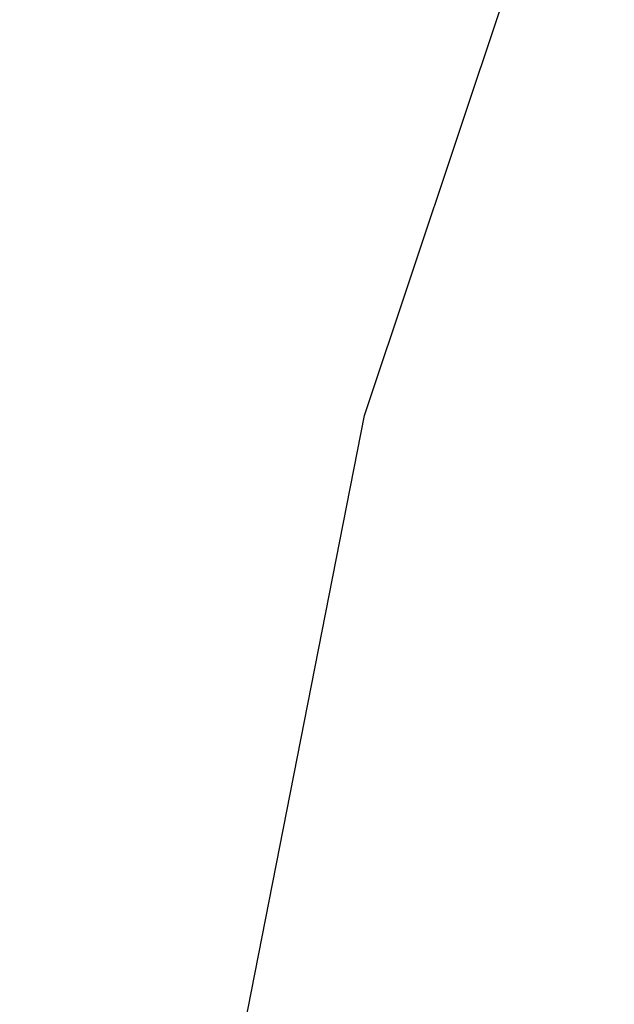
# Model space of a CAD drawing. Units: inches. Extents: x 3590 to 5167, y 65 to 1917.
# Tile 81 of 100: x 5050.9101 to 5051.162, y 1788.6144 to 1789.0318. Entities that reach past the tile are written whole.
import ezdxf

# ---------------------------------------------------------------- set-up
doc = ezdxf.new("R2010")
doc.units = ezdxf.units.IN
for name, color, linetype, lineweight in [('A-ANNO-DIMS', 2, 'Continuous', 18), ('A-FLOR-PATT', 8, 'Continuous', 13), ('L-PLNT', 94, 'Continuous', 18)]:
    doc.layers.add(name, color=color, linetype=linetype, lineweight=lineweight)
doc.layers.add('DIENHOA', color=3, linetype='Continuous')
doc.styles.get("Standard").update_dxf_attribs({"font": 'arial.ttf'})
doc.dimstyles.new('ISO-25', dxfattribs={"dimtxt": 9, "dimasz": 2.5, "dimexe": 1.25, "dimexo": 0.625, "dimtad": 1, "dimdec": 1, "dimlunit": 3, "dimtxsty": 'Standard', "dimcen": 2.5, "dimadec": 0, "dimazin": 0, "dimtfac": 1, "dimtdec": 1, "dimtmove": 0, "dimatfit": 3, "dimfxl": 1, "dimarcsym": 0})

# ---------------------------------------------------------------- blocks, each defined once
blk = doc.blocks.new('Cay03_mb')
at = {"layer": 'DIENHOA'}
for p, q in [((25.486, 374.333), (48.564, 443.581)), ((9.944, 295.252), (25.486, 374.333))]:
    blk.add_line(p, q, dxfattribs=at)
blk = doc.blocks.new('*D323')
at = {"layer": 'A-ANNO-DIMS', "color": 0, "lineweight": -2, "transparency": 16777216}
for p, q in [((5069.17227, 1795.21603), (5069.17227, 1874.95034)), ((5065.43703, 1795.21603), (5070.42227, 1795.21603)), ((5069.17227, 1769.30924), (5069.17227, 1792.71603)), ((5065.43703, 1766.80924), (5070.42227, 1766.80924))]:
    blk.add_line(p, q, dxfattribs=at)
at = {"layer": 'A-ANNO-DIMS', "color": 0, "transparency": 16777216}
for points in [[(5068.75561, 1792.71603), (5069.58894, 1792.71603), (5069.17227, 1795.21603)], [(5068.75561, 1769.30924), (5069.58894, 1769.30924), (5069.17227, 1766.80924)]]:
    blk.add_solid(points, dxfattribs=at)
at = {"layer": 'Defpoints', "color": 0, "transparency": 16777216}
for p in [(5064.81203, 1795.21603), (5069.17227, 1795.21603), (5064.81203, 1766.80924)]:
    blk.add_point(p, dxfattribs=at)
at = {"layer": 'A-ANNO-DIMS', "color": 0, "transparency": 16777216, "insert": (5063.89379, 1836.33318), "char_height": 9, "attachment_point": 5, "rotation": 90}
blk.add_mtext('2\'-4 1/2" TYP.', dxfattribs=at)

msp = doc.modelspace()

# ---------------------------------------------------------------- hatches: boundary and pattern name
at = {"layer": 'A-FLOR-PATT', "transparency": 33554687}
h = msp.add_hatch(dxfattribs=at)
h.set_pattern_fill('AR-HBONE', color=256, scale=0.2)
h.set_pattern_definition([(45, (-588.972, 0), (0, 28.73682), [60.96, -20.32]), (135, (-574.604, 14.368), (3e-15, 28.73682), [60.96, -20.32])])
h.paths.add_polyline_path([(5071.27403, 1796.99898), (4933.27403, 1796.99898), (4933.27403, 1753.99898), (4962.77403, 1753.99898, -0.414214), (4928.77403, 1719.99898), (4933.27403, 1718.99898), (4933.27403, 1334.99898), (5071.27403, 1334.99898)])
h.paths.add_polyline_path([(4951.78002, 1521.0767), (4951.7151, 1521.0404), (4951.56345, 1520.89532)], flags=16)
h.paths.add_polyline_path([(4952.267, 1521.37645), (4952.1977, 1521.37111), (4952.19823, 1521.35558)], flags=0)
h.paths.add_polyline_path([(4967.05076, 1529.72832), (4965.23122, 1528.69444), (4963.41109, 1527.71401), (4961.75649, 1526.85081), (4963.58887, 1527.44938), (4964.03555, 1527.47802), (4962.9755, 1527.24902), (4961.76022, 1526.85203), (4959.79219, 1525.83406), (4958.00498, 1524.89483), (4956.24031, 1523.92961), (4954.50395, 1522.91854), (4954.1294, 1522.68163), (4953.36051, 1521.99688), (4953.36558, 1521.99754), (4953.605, 1522.06367), (4955.10605, 1522.76083), (4956.92108, 1523.43405), (4958.67784, 1523.91513), (4960.35834, 1524.20036), (4961.94456, 1524.28606), (4964.17144, 1524.10849), (4965.95752, 1523.30903), (4963.86273, 1522.97565), (4965.18742, 1522.49898), (4963.36614, 1522.49715), (4961.54526, 1522.48682), (4959.76359, 1522.46077), (4958.30414, 1522.4188), (4957.97356, 1522.38829), (4956.30692, 1522.2324), (4954.71821, 1522.07143), (4953.25077, 1521.89915), (4953.52509, 1521.62277), (4954.33087, 1521.37883), (4956.24263, 1521.22987), (4958.03913, 1520.92952), (4959.68424, 1520.48339), (4961.16007, 1519.89569), (4963.10699, 1518.80022), (4964.39286, 1517.32518), (4962.97306, 1517.72596), (4964.55841, 1516.66059), (4965.40664, 1515.70779), (4963.50733, 1516.32179), (4961.67995, 1517.0051), (4959.93478, 1517.74489), (4958.2821, 1518.52833), (4956.73216, 1519.34257), (4955.29527, 1520.17478), (4954.67155, 1520.57237), (4954.51279, 1520.6271), (4955.65848, 1519.31837), (4956.70263, 1517.98232), (4957.64403, 1516.64663), (4958.48545, 1515.33439), (4959.54998, 1513.52398), (4960.43768, 1511.76936), (4958.84107, 1513.6196), (4957.45175, 1515.3249), (4955.8186, 1517.45855), (4956.66537, 1515.44764), (4957.11109, 1513.92292), (4957.44681, 1511.71434), (4957.07641, 1509.79288), (4956.53757, 1511.1103), (4955.99231, 1512.56892), (4955.44448, 1514.12509), (4954.89794, 1515.73518), (4954.35653, 1517.35553), (4953.82412, 1518.94251), (4953.30455, 1520.45247), (4953.06452, 1521.11563), (4952.97143, 1521.14607), (4952.94932, 1521.08646), (4952.72981, 1520.19905), (4953.3698, 1518.02364), (4953.75708, 1516.37279), (4954.05124, 1514.76538), (4954.26449, 1513.22121), (4954.47124, 1511.13121), (4954.4971, 1510.40174), (4954.40903, 1511.76006), (4954.26449, 1513.22121), (4954.05124, 1514.76538), (4953.75708, 1516.37279), (4953.3698, 1518.02364), (4952.87718, 1519.69813), (4952.7161, 1520.1412), (4952.53301, 1519.05871), (4952.37428, 1517.78881), (4952.21925, 1516.31167), (4952.04598, 1514.59986), (4951.83253, 1512.62598), (4951.55697, 1510.36259), (4951.20331, 1512.16818), (4950.85168, 1514.33931), (4950.98529, 1516.37594), (4951.6596, 1518.28625), (4952.59261, 1520.48085), (4952.35664, 1521.1299), (4951.85502, 1520.32753), (4950.83901, 1518.90828), (4949.77675, 1517.58658), (4948.91554, 1516.61731), (4948.11099, 1515.2561), (4947.0891, 1513.55389), (4945.88937, 1511.61495), (4946.32587, 1513.40232), (4946.5624, 1514.24913), (4945.52771, 1513.32668), (4944.58105, 1512.53126), (4946.01774, 1514.50825), (4947.2044, 1516.04763), (4947.89331, 1517.31331), (4949.30686, 1518.76446), (4950.41417, 1519.76716), (4950.45131, 1519.80628), (4952.267, 1521.37645), (4951.64457, 1521.49317), (4950.40371, 1521.17954), (4948.04447, 1520.35868), (4946.11863, 1519.45198), (4944.57182, 1518.47484), (4943.34962, 1517.44265), (4941.99695, 1515.91971), (4941.66146, 1515.27475), (4942.81332, 1516.98973), (4944.57182, 1518.47484), (4946.11863, 1519.45198), (4948.04447, 1520.35868), (4950.40371, 1521.17954), (4951.64457, 1521.49317), (4949.64678, 1521.86781), (4948.59979, 1521.75633), (4947.12629, 1521.5699), (4945.42015, 1521.34763), (4943.44969, 1521.10462), (4941.18319, 1520.85596), (4942.86028, 1521.61265), (4943.87308, 1522.03014), (4942.95216, 1521.9093), (4941.40968, 1521.48512), (4939.54287, 1520.67019), (4938.96775, 1520.2255), (4940.73284, 1521.29899), (4942.95216, 1521.9093), (4943.70184, 1522.00767), (4945.89419, 1522.69998), (4947.56488, 1522.71399), (4948.92086, 1522.56573), (4951.13144, 1522.18271), (4950.97062, 1522.2969), (4948.12924, 1523.00563), (4946.03496, 1523.70671), (4944.23235, 1524.52143), (4942.70692, 1525.46111), (4941.44419, 1526.53707), (4940.42968, 1527.76062), (4939.6489, 1529.14306), (4941.42091, 1528.12232), (4943.14742, 1527.13248), (4944.84093, 1526.17457), (4946.51394, 1525.24959), (4948.17893, 1524.35855), (4948.36457, 1524.26336), (4946.47531, 1526.04459), (4945.18083, 1527.54042), (4944.19039, 1529.03339), (4943.49559, 1530.53985), (4943.27808, 1531.3597), (4942.49849, 1531.91903), (4943.11353, 1531.76249), (4942.95927, 1533.6586), (4944.13953, 1531.9886), (4944.61171, 1531.32339), (4946.20163, 1530.46341), (4947.48567, 1529.50925), (4948.79027, 1528.22649), (4950.36754, 1526.23746), (4949.48547, 1528.15549), (4948.85128, 1530.12254), (4948.49054, 1532.04127), (4948.38105, 1533.91822), (4948.50062, 1535.7599), (4948.82704, 1537.57284), (4949.41803, 1535.56526), (4949.95684, 1533.56932), (4950.46414, 1531.5861), (4950.96058, 1529.6167), (4951.3911, 1527.95448), (4951.72352, 1530.68689), (4952.20106, 1532.57994), (4952.88914, 1534.32964), (4953.77035, 1535.95123), (4954.82726, 1537.45995), (4954.52145, 1535.38966), (4954.27314, 1533.93684), (4955.57999, 1535.6627), (4956.74758, 1536.73859), (4956.15852, 1534.78029), (4955.58917, 1532.87334), (4955.04336, 1531.00581), (4954.52493, 1529.16576), (4954.03771, 1527.34127), (4953.63833, 1525.73298), (4953.61143, 1525.58564), (4953.39805, 1524.16565), (4953.38219, 1524.00887), (4954.06955, 1525.47563), (4954.91212, 1527.02173), (4956.13627, 1528.89351), (4957.84668, 1530.57701), (4959.37601, 1531.54014), (4958.25596, 1530.10398), (4957.14284, 1528.66291), (4956.06626, 1527.24305), (4955.05579, 1525.87054), (4954.14104, 1524.57149), (4953.35159, 1523.37204), (4953.31079, 1523.30299), (4953.27253, 1522.92478), (4953.26102, 1522.38213), (4954.1031, 1523.37273), (4954.63005, 1524.28376), (4955.96149, 1526.35767), (4957.23002, 1528.12969), (4958.42057, 1529.60864), (4960.03671, 1531.36792), (4961.3736, 1532.3752), (4962.1015, 1532.77), (4961.06994, 1531.06113), (4959.98733, 1529.43811), (4958.86851, 1527.90803), (4958.15046, 1527.00742), (4959.80291, 1528.00314), (4961.58854, 1528.79257), (4963.39087, 1529.32783), (4965.21118, 1529.63205)], flags=16)
h.paths.add_polyline_path([(4962.94387, 1523.18187), (4961.10714, 1523.42192), (4960.39205, 1523.36158), (4962.34964, 1523.33061)], flags=0)
h.paths.add_polyline_path([(5049.54129, 1584.55089), (5049.47636, 1584.51458), (5049.32471, 1584.3695)], flags=16)
h.paths.add_polyline_path([(5050.02827, 1584.85063), (5049.95897, 1584.84529), (5049.95949, 1584.82976)], flags=0)
h.paths.add_polyline_path([(5042.33308, 1581.94902), (5043.8799, 1582.92616), (5045.80573, 1583.83286), (5048.16498, 1584.65372), (5049.40583, 1584.96736), (5047.40804, 1585.34199), (5046.36106, 1585.23052), (5044.88755, 1585.04408), (5043.18142, 1584.82181), (5041.21095, 1584.5788), (5038.94446, 1584.33014), (5040.62155, 1585.08683), (5041.63434, 1585.50432), (5040.71343, 1585.38348), (5039.17095, 1584.9593), (5037.30414, 1584.14438), (5036.72901, 1583.69969), (5038.4941, 1584.77317), (5040.71343, 1585.38348), (5041.4631, 1585.48185), (5043.65545, 1586.17416), (5045.32615, 1586.18818), (5046.68212, 1586.03992), (5048.8927, 1585.6569), (5048.73188, 1585.77108), (5045.89051, 1586.47981), (5043.79622, 1587.18089), (5041.99361, 1587.99561), (5040.46818, 1588.9353), (5039.20546, 1590.01125), (5038.19095, 1591.2348), (5037.41016, 1592.61725), (5039.18217, 1591.5965), (5040.90868, 1590.60667), (5042.6022, 1589.64876), (5044.2752, 1588.72378), (5045.94019, 1587.83274), (5046.12584, 1587.73754), (5044.23658, 1589.51878), (5042.9421, 1591.01461), (5041.95166, 1592.50757), (5041.25685, 1594.01403), (5041.03935, 1594.83388), (5040.25976, 1595.39321), (5040.8748, 1595.23667), (5040.72054, 1597.13279), (5041.9008, 1595.46278), (5042.37297, 1594.79758), (5043.96289, 1593.93759), (5045.24694, 1592.98344), (5046.55153, 1591.70068), (5048.12881, 1589.71164), (5047.24673, 1591.62967), (5046.61254, 1593.59672), (5046.2518, 1595.51546), (5046.14232, 1597.3924), (5046.26189, 1599.23408), (5046.5883, 1601.04703), (5047.17929, 1599.03944), (5047.71811, 1597.0435), (5048.22541, 1595.06028), (5048.72184, 1593.09089), (5049.15237, 1591.42866), (5049.48478, 1594.16107), (5049.96233, 1596.05412), (5050.65041, 1597.80382), (5051.53161, 1599.42541), (5052.58852, 1600.93414), (5052.28271, 1598.86384), (5052.03441, 1597.41102), (5053.34126, 1599.13689), (5054.50884, 1600.21277), (5053.91979, 1598.25447), (5053.35044, 1596.34752), (5052.80463, 1594.47999), (5052.2862, 1592.63995), (5051.79898, 1590.81546), (5051.39959, 1589.20716), (5051.3727, 1589.05983), (5051.15931, 1587.63984), (5051.14346, 1587.48305), (5051.83082, 1588.94982), (5052.67339, 1590.49592), (5053.89754, 1592.3677), (5055.60794, 1594.05119), (5057.13728, 1595.01432), (5056.01722, 1593.57817), (5054.90411, 1592.1371), (5053.82752, 1590.71724), (5052.81705, 1589.34472), (5051.9023, 1588.04567), (5051.11286, 1586.84622), (5051.07205, 1586.77718), (5051.03379, 1586.39896), (5051.02228, 1585.85631), (5051.86437, 1586.84692), (5052.39131, 1587.75794), (5053.72275, 1589.83185), (5054.99128, 1591.60387), (5056.18183, 1593.08282), (5057.79798, 1594.84211), (5059.13486, 1595.84938), (5059.86276, 1596.24419), (5058.83121, 1594.53531), (5057.7486, 1592.9123), (5056.62978, 1591.38221), (5055.91173, 1590.4816), (5057.56418, 1591.47732), (5059.34981, 1592.26675), (5061.15214, 1592.80202), (5062.97245, 1593.10624), (5064.81203, 1593.20251), (5062.99248, 1592.16863), (5061.17235, 1591.18819), (5059.51775, 1590.325), (5061.35014, 1590.92356), (5061.79682, 1590.95221), (5060.73676, 1590.7232), (5059.52148, 1590.32622), (5057.55345, 1589.30825), (5055.76625, 1588.36901), (5054.00157, 1587.40379), (5052.26521, 1586.39273), (5051.89067, 1586.15581), (5051.12177, 1585.47106), (5051.12684, 1585.47172), (5051.36627, 1585.53786), (5052.86732, 1586.23502), (5054.68234, 1586.90824), (5056.4391, 1587.38931), (5058.1196, 1587.67454), (5059.70582, 1587.76024), (5061.93271, 1587.58268), (5063.71878, 1586.78321), (5061.62399, 1586.44983), (5062.94869, 1585.97317), (5061.12741, 1585.97133), (5059.30653, 1585.961), (5057.52486, 1585.93496), (5056.06541, 1585.89299), (5055.73482, 1585.86247), (5054.06819, 1585.70658), (5052.47947, 1585.54561), (5051.01204, 1585.37333), (5051.28635, 1585.09695), (5052.09214, 1584.85301), (5054.00389, 1584.70406), (5055.8004, 1584.4037), (5057.44551, 1583.95757), (5058.92133, 1583.36987), (5060.86825, 1582.27441), (5062.15413, 1580.79937), (5060.73433, 1581.20015), (5062.31967, 1580.13477), (5063.1679, 1579.18198), (5061.2686, 1579.79597), (5059.44122, 1580.47928), (5057.69605, 1581.21908), (5056.04336, 1582.00251), (5054.49343, 1582.81675), (5053.05653, 1583.64897), (5052.43281, 1584.04656), (5052.27405, 1584.10128), (5053.41974, 1582.79255), (5054.4639, 1581.4565), (5055.40529, 1580.12081), (5056.24672, 1578.80858), (5057.31125, 1576.99816), (5058.19895, 1575.24354), (5056.60234, 1577.09378), (5055.21301, 1578.79908), (5053.57987, 1580.93274), (5054.42664, 1578.92183), (5054.87235, 1577.3971), (5055.20808, 1575.18852), (5054.83767, 1573.26706), (5054.29883, 1574.58448), (5053.75357, 1576.0431), (5053.20575, 1577.59927), (5052.6592, 1579.20936), (5052.1178, 1580.82971), (5051.58538, 1582.41669), (5051.06582, 1583.92666), (5050.82578, 1584.58981), (5050.7327, 1584.62025), (5050.71058, 1584.56064), (5050.49108, 1583.67323), (5051.13107, 1581.49782), (5051.51835, 1579.84698), (5051.8125, 1578.23957), (5052.02575, 1576.69539), (5052.23251, 1574.6054), (5052.25836, 1573.87593), (5052.1703, 1575.23424), (5052.02575, 1576.69539), (5051.8125, 1578.23957), (5051.51835, 1579.84698), (5051.13107, 1581.49782), (5050.63844, 1583.17231), (5050.47736, 1583.61538), (5050.29428, 1582.53289), (5050.13554, 1581.26299), (5049.98051, 1579.78585), (5049.80724, 1578.07405), (5049.59379, 1576.10016), (5049.31823, 1573.83678), (5048.96458, 1575.64237), (5048.61294, 1577.8135), (5048.74656, 1579.85012), (5049.42086, 1581.76043), (5050.35388, 1583.95503), (5050.1179, 1584.60408), (5049.61629, 1583.80172), (5048.60027, 1582.38246), (5047.53801, 1581.06076), (5046.67681, 1580.09149), (5045.87225, 1578.73029), (5044.85036, 1577.02808), (5043.65063, 1575.08913), (5044.08713, 1576.8765), (5044.32366, 1577.72331), (5043.28898, 1576.80086), (5042.34232, 1576.00545), (5043.779, 1577.98243), (5044.96566, 1579.52182), (5045.65457, 1580.78749), (5047.06813, 1582.23865), (5048.17543, 1583.24134), (5048.21258, 1583.28047), (5050.02827, 1584.85063), (5049.40583, 1584.96736), (5048.16498, 1584.65372), (5045.80573, 1583.83286), (5043.8799, 1582.92616), (5042.33308, 1581.94902), (5041.11088, 1580.91684), (5039.75821, 1579.39389), (5039.42272, 1578.74894), (5040.57458, 1580.46391)], flags=16)
h.paths.add_polyline_path([(4954.79872, 1533.12029), (4954.26249, 1532.07935), (4953.83112, 1530.93464), (4953.50472, 1529.63602), (4953.28338, 1528.13331), (4953.16721, 1526.37637), (4953.15631, 1524.31504), (4953.27669, 1521.23629), (4952.80168, 1521.84177), (4951.55695, 1521.99789), (4950.97575, 1521.9613), (4952.66059, 1521.94097), (4952.80168, 1521.84177), (4953.15249, 1523.59258), (4953.16721, 1526.37637), (4953.28338, 1528.13331), (4953.60929, 1530.34598), (4954.45558, 1532.59174)], flags=0)
h.paths.add_polyline_path([(5050.56294, 1585.31596), (5049.31822, 1585.47208), (5048.73702, 1585.43548), (5050.42186, 1585.41516), (5050.56294, 1585.31596), (5050.91375, 1587.06676), (5050.92848, 1589.85056), (5051.04465, 1591.6075), (5051.37055, 1593.82017), (5052.21684, 1596.06593), (5052.55999, 1596.59447), (5052.02375, 1595.55353), (5051.59238, 1594.40883), (5051.26598, 1593.1102), (5051.04465, 1591.6075), (5050.92848, 1589.85056), (5050.91757, 1587.78922), (5051.03795, 1584.71048)], flags=0)
h.paths.add_polyline_path([(5058.15332, 1586.83576), (5060.11091, 1586.80479), (5060.70514, 1586.65605), (5058.8684, 1586.8961)], flags=0)
h.paths.add_polyline_path([(5049.54129, 1430.93611), (5049.47636, 1430.8998), (5049.32471, 1430.75472)], flags=16)
h.paths.add_polyline_path([(5050.02827, 1431.23585), (5049.95897, 1431.23051), (5049.95949, 1431.21498)], flags=0)
h.paths.add_polyline_path([(5046.5883, 1447.43225), (5047.17929, 1445.42467), (5047.71811, 1443.42872), (5048.22541, 1441.4455), (5048.72184, 1439.47611), (5049.15237, 1437.81388), (5049.48478, 1440.5463), (5049.96233, 1442.43934), (5050.65041, 1444.18904), (5051.53161, 1445.81063), (5052.58852, 1447.31936), (5052.28271, 1445.24906), (5052.03441, 1443.79624), (5053.34126, 1445.52211), (5054.50884, 1446.59799), (5053.91979, 1444.63969), (5053.35044, 1442.73274), (5052.80463, 1440.86521), (5052.2862, 1439.02517), (5051.79898, 1437.20068), (5051.39959, 1435.59238), (5051.3727, 1435.44505), (5051.15931, 1434.02506), (5051.14346, 1433.86828), (5051.83082, 1435.33504), (5052.67339, 1436.88114), (5053.89754, 1438.75292), (5055.60794, 1440.43641), (5057.13728, 1441.39954), (5056.01722, 1439.96339), (5054.90411, 1438.52232), (5053.82752, 1437.10246), (5052.81705, 1435.72994), (5051.9023, 1434.4309), (5051.11286, 1433.23145), (5051.07205, 1433.1624), (5051.03379, 1432.78418), (5051.02228, 1432.24153), (5051.86437, 1433.23214), (5052.39131, 1434.14316), (5053.72275, 1436.21707), (5054.99128, 1437.98909), (5056.18183, 1439.46805), (5057.79798, 1441.22733), (5059.13486, 1442.23461), (5059.86276, 1442.62941), (5058.83121, 1440.92053), (5057.7486, 1439.29752), (5056.62978, 1437.76743), (5055.91173, 1436.86682), (5057.56418, 1437.86255), (5059.34981, 1438.65197), (5061.15214, 1439.18724), (5062.97245, 1439.49146), (5064.81203, 1439.58773), (5062.99248, 1438.55385), (5061.17235, 1437.57342), (5059.51775, 1436.71022), (5061.35014, 1437.30879), (5061.79682, 1437.33743), (5060.73676, 1437.10842), (5059.52148, 1436.71144), (5057.55345, 1435.69347), (5055.76625, 1434.75423), (5054.00157, 1433.78901), (5052.26521, 1432.77795), (5051.89067, 1432.54103), (5051.12177, 1431.85628), (5051.12684, 1431.85694), (5051.36627, 1431.92308), (5052.86732, 1432.62024), (5054.68234, 1433.29346), (5056.4391, 1433.77453), (5058.1196, 1434.05976), (5059.70582, 1434.14546), (5061.93271, 1433.9679), (5063.71878, 1433.16843), (5061.62399, 1432.83505), (5062.94869, 1432.35839), (5061.12741, 1432.35655), (5059.30653, 1432.34623), (5057.52486, 1432.32018), (5056.06541, 1432.27821), (5055.73482, 1432.24769), (5054.06819, 1432.09181), (5052.47947, 1431.93083), (5051.01204, 1431.75856), (5051.28635, 1431.48218), (5052.09214, 1431.23823), (5054.00389, 1431.08928), (5055.8004, 1430.78892), (5057.44551, 1430.34279), (5058.92133, 1429.75509), (5060.86825, 1428.65963), (5062.15413, 1427.18459), (5060.73433, 1427.58537), (5062.31967, 1426.52), (5063.1679, 1425.5672), (5061.2686, 1426.18119), (5059.44122, 1426.86451), (5057.69605, 1427.6043), (5056.04336, 1428.38773), (5054.49343, 1429.20197), (5053.05653, 1430.03419), (5052.43281, 1430.43178), (5052.27405, 1430.48651), (5053.41974, 1429.17777), (5054.4639, 1427.84172), (5055.40529, 1426.50603), (5056.24672, 1425.1938), (5057.31125, 1423.38338), (5058.19895, 1421.62877), (5056.60234, 1423.479), (5055.21301, 1425.1843), (5053.57987, 1427.31796), (5054.42664, 1425.30705), (5054.87235, 1423.78233), (5055.20808, 1421.57374), (5054.83767, 1419.65228), (5054.29883, 1420.9697), (5053.75357, 1422.42832), (5053.20575, 1423.9845), (5052.6592, 1425.59458), (5052.1178, 1427.21493), (5051.58538, 1428.80191), (5051.06582, 1430.31188), (5050.82578, 1430.97503), (5050.7327, 1431.00547), (5050.71058, 1430.94586), (5050.49108, 1430.05845), (5051.13107, 1427.88305), (5051.51835, 1426.2322), (5051.8125, 1424.62479), (5052.02575, 1423.08061), (5052.23251, 1420.99062), (5052.25836, 1420.26115), (5052.1703, 1421.61947), (5052.02575, 1423.08061), (5051.8125, 1424.62479), (5051.51835, 1426.2322), (5051.13107, 1427.88305), (5050.63844, 1429.55753), (5050.47736, 1430.0006), (5050.29428, 1428.91811), (5050.13554, 1427.64821), (5049.98051, 1426.17107), (5049.80724, 1424.45927), (5049.59379, 1422.48539), (5049.31823, 1420.222), (5048.96458, 1422.02759), (5048.61294, 1424.19872), (5048.74656, 1426.23534), (5049.42086, 1428.14565), (5050.35388, 1430.34025), (5050.1179, 1430.98931), (5049.61629, 1430.18694), (5048.60027, 1428.76768), (5047.53801, 1427.44598), (5046.67681, 1426.47671), (5045.87225, 1425.11551), (5044.85036, 1423.4133), (5043.65063, 1421.47435), (5044.08713, 1423.26172), (5044.32366, 1424.10854), (5043.28898, 1423.18608), (5042.34232, 1422.39067), (5043.779, 1424.36765), (5044.96566, 1425.90704), (5045.65457, 1427.17272), (5047.06813, 1428.62387), (5048.17543, 1429.62657), (5048.21258, 1429.66569), (5050.02827, 1431.23585), (5049.40583, 1431.35258), (5048.16498, 1431.03894), (5045.80573, 1430.21809), (5043.8799, 1429.31139), (5042.33308, 1428.33424), (5041.11088, 1427.30206), (5039.75821, 1425.77911), (5039.42272, 1425.13416), (5040.57458, 1426.84914), (5042.33308, 1428.33424), (5043.8799, 1429.31139), (5045.80573, 1430.21809), (5048.16498, 1431.03894), (5049.40583, 1431.35258), (5047.40804, 1431.72722), (5046.36106, 1431.61574), (5044.88755, 1431.42931), (5043.18142, 1431.20704), (5041.21095, 1430.96402), (5038.94446, 1430.71536), (5040.62155, 1431.47205), (5041.63434, 1431.88954), (5040.71343, 1431.76871), (5039.17095, 1431.34453), (5037.30414, 1430.5296), (5036.72901, 1430.08491), (5038.4941, 1431.1584), (5040.71343, 1431.76871), (5041.4631, 1431.86707), (5043.65545, 1432.55939), (5045.32615, 1432.5734), (5046.68212, 1432.42514), (5048.8927, 1432.04212), (5048.73188, 1432.1563), (5045.89051, 1432.86503), (5043.79622, 1433.56611), (5041.99361, 1434.38083), (5040.46818, 1435.32052), (5039.20546, 1436.39648), (5038.19095, 1437.62002), (5037.41016, 1439.00247), (5039.18217, 1437.98172), (5040.90868, 1436.99189), (5042.6022, 1436.03398), (5044.2752, 1435.109), (5045.94019, 1434.21796), (5046.12584, 1434.12276), (5044.23658, 1435.904), (5042.9421, 1437.39983), (5041.95166, 1438.8928), (5041.25685, 1440.39925), (5041.03935, 1441.2191), (5040.25976, 1441.77844), (5040.8748, 1441.62189), (5040.72054, 1443.51801), (5041.9008, 1441.848), (5042.37297, 1441.1828), (5043.96289, 1440.32282), (5045.24694, 1439.36866), (5046.55153, 1438.0859), (5048.12881, 1436.09686), (5047.24673, 1438.01489), (5046.61254, 1439.98195), (5046.2518, 1441.90068), (5046.14232, 1443.77762), (5046.26189, 1445.6193)], flags=16)
h.paths.add_polyline_path([(5052.38176, 1444.25496), (5051.62263, 1442.77987), (5052.02375, 1441.93875), (5052.55999, 1442.9797)], flags=0)
h.paths.add_polyline_path([(5050.56294, 1431.70118), (5049.31822, 1431.8573), (5048.73702, 1431.82071), (5050.42186, 1431.80038)], flags=0)
h.paths.add_polyline_path([(5058.15332, 1433.22098), (5060.11091, 1433.19001), (5060.70514, 1433.04127), (5058.8684, 1433.28132)], flags=0)
h.paths.add_polyline_path([(5049.54129, 1352.28535), (5049.47636, 1352.24904), (5049.32471, 1352.10396)], flags=16)
h.paths.add_polyline_path([(5050.02827, 1352.58509), (5049.95897, 1352.57975), (5049.95949, 1352.56422)], flags=0)
h.paths.add_polyline_path([(5046.5883, 1368.78149), (5047.17929, 1366.7739), (5047.71811, 1364.77796), (5048.22541, 1362.79474), (5048.72184, 1360.82534), (5049.15237, 1359.16312), (5049.48478, 1361.89553), (5049.96233, 1363.78858), (5050.65041, 1365.53828), (5051.53161, 1367.15987), (5052.58852, 1368.6686), (5052.28271, 1366.5983), (5052.03441, 1365.14548), (5053.34126, 1366.87135), (5054.50884, 1367.94723), (5053.91979, 1365.98893), (5053.35044, 1364.08198), (5052.80463, 1362.21445), (5052.2862, 1360.37441), (5051.79898, 1358.54992), (5051.39959, 1356.94162), (5051.3727, 1356.79428), (5051.15931, 1355.37429), (5051.14346, 1355.21751), (5051.83082, 1356.68428), (5052.67339, 1358.23037), (5053.89754, 1360.10216), (5055.60794, 1361.78565), (5057.13728, 1362.74878), (5056.01722, 1361.31262), (5054.90411, 1359.87155), (5053.82752, 1358.4517), (5052.81705, 1357.07918), (5051.9023, 1355.78013), (5051.11286, 1354.58068), (5051.07205, 1354.51164), (5051.03379, 1354.13342), (5051.02228, 1353.59077), (5051.86437, 1354.58137), (5052.39131, 1355.4924), (5053.72275, 1357.56631), (5054.99128, 1359.33833), (5056.18183, 1360.81728), (5057.79798, 1362.57656), (5059.13486, 1363.58384), (5059.86276, 1363.97864), (5058.83121, 1362.26977), (5057.7486, 1360.64675), (5056.62978, 1359.11667), (5055.91173, 1358.21606), (5057.56418, 1359.21178), (5059.34981, 1360.00121), (5061.15214, 1360.53648), (5062.97245, 1360.84069), (5064.81203, 1360.93697), (5062.99248, 1359.90308), (5061.17235, 1358.92265), (5059.51775, 1358.05946), (5061.35014, 1358.65802), (5061.79682, 1358.68666), (5060.73676, 1358.45766), (5059.52148, 1358.06068), (5057.55345, 1357.0427), (5055.76625, 1356.10347), (5054.00157, 1355.13825), (5052.26521, 1354.12718), (5051.89067, 1353.89027), (5051.12177, 1353.20552), (5051.12684, 1353.20618), (5051.36627, 1353.27231), (5052.86732, 1353.96947), (5054.68234, 1354.6427), (5056.4391, 1355.12377), (5058.1196, 1355.409), (5059.70582, 1355.4947), (5061.93271, 1355.31713), (5063.71878, 1354.51767), (5061.62399, 1354.18429), (5062.94869, 1353.70763), (5061.12741, 1353.70579), (5059.30653, 1353.69546), (5057.52486, 1353.66942), (5056.06541, 1353.62744), (5055.73482, 1353.59693), (5054.06819, 1353.44104), (5052.47947, 1353.28007), (5051.01204, 1353.10779), (5051.28635, 1352.83141), (5052.09214, 1352.58747), (5054.00389, 1352.43852), (5055.8004, 1352.13816), (5057.44551, 1351.69203), (5058.92133, 1351.10433), (5060.86825, 1350.00887), (5062.15413, 1348.53382), (5060.73433, 1348.9346), (5062.31967, 1347.86923), (5063.1679, 1346.91643), (5061.2686, 1347.53043), (5059.44122, 1348.21374), (5057.69605, 1348.95353), (5056.04336, 1349.73697), (5054.49343, 1350.55121), (5053.05653, 1351.38342), (5052.43281, 1351.78101), (5052.27405, 1351.83574), (5053.41974, 1350.52701), (5054.4639, 1349.19096), (5055.40529, 1347.85527), (5056.24672, 1346.54303), (5057.31125, 1344.73262), (5058.19895, 1342.978), (5056.60234, 1344.82824), (5055.21301, 1346.53354), (5053.57987, 1348.6672), (5054.42664, 1346.65629), (5054.87235, 1345.13156), (5055.20808, 1342.92298), (5054.83767, 1341.00152), (5054.29883, 1342.31894), (5053.75357, 1343.77756), (5053.20575, 1345.33373), (5052.6592, 1346.94382), (5052.1178, 1348.56417), (5051.58538, 1350.15115), (5051.06582, 1351.66111), (5050.82578, 1352.32427), (5050.7327, 1352.35471), (5050.71058, 1352.2951), (5050.49108, 1351.40769), (5051.13107, 1349.23228), (5051.51835, 1347.58144), (5051.8125, 1345.97403), (5052.02575, 1344.42985), (5052.23251, 1342.33986), (5052.25836, 1341.61039), (5052.1703, 1342.9687), (5052.02575, 1344.42985), (5051.8125, 1345.97403), (5051.51835, 1347.58144), (5051.13107, 1349.23228), (5050.63844, 1350.90677), (5050.47736, 1351.34984), (5050.29428, 1350.26735), (5050.13554, 1348.99745), (5049.98051, 1347.52031), (5049.80724, 1345.80851), (5049.59379, 1343.83462), (5049.31823, 1341.57124), (5048.96458, 1343.37683), (5048.61294, 1345.54796), (5048.74656, 1347.58458), (5049.42086, 1349.49489), (5050.35388, 1351.68949), (5050.1179, 1352.33854), (5049.61629, 1351.53617), (5048.60027, 1350.11692), (5047.53801, 1348.79522), (5046.67681, 1347.82595), (5045.87225, 1346.46475), (5044.85036, 1344.76253), (5043.65063, 1342.82359), (5044.08713, 1344.61096), (5044.32366, 1345.45777), (5043.28898, 1344.53532), (5042.34232, 1343.7399), (5043.779, 1345.71689), (5044.96566, 1347.25627), (5045.65457, 1348.52195), (5047.06813, 1349.9731), (5048.17543, 1350.9758), (5048.21258, 1351.01493), (5050.02827, 1352.58509), (5049.40583, 1352.70181), (5048.16498, 1352.38818), (5045.80573, 1351.56732), (5043.8799, 1350.66062), (5042.33308, 1349.68348), (5041.11088, 1348.65129), (5039.75821, 1347.12835), (5039.42272, 1346.4834), (5040.57458, 1348.19837), (5042.33308, 1349.68348), (5043.8799, 1350.66062), (5045.80573, 1351.56732), (5048.16498, 1352.38818), (5049.40583, 1352.70181), (5047.40804, 1353.07645), (5046.36106, 1352.96498), (5044.88755, 1352.77854), (5043.18142, 1352.55627), (5041.21095, 1352.31326), (5038.94446, 1352.0646), (5040.62155, 1352.82129), (5041.63434, 1353.23878), (5040.71343, 1353.11794), (5039.17095, 1352.69376), (5037.30414, 1351.87884), (5036.72901, 1351.43415), (5038.4941, 1352.50763), (5040.71343, 1353.11794), (5041.4631, 1353.21631), (5043.65545, 1353.90862), (5045.32615, 1353.92263), (5046.68212, 1353.77438), (5048.8927, 1353.39136), (5048.73188, 1353.50554), (5045.89051, 1354.21427), (5043.79622, 1354.91535), (5041.99361, 1355.73007), (5040.46818, 1356.66975), (5039.20546, 1357.74571), (5038.19095, 1358.96926), (5037.41016, 1360.35171), (5039.18217, 1359.33096), (5040.90868, 1358.34112), (5042.6022, 1357.38321), (5044.2752, 1356.45824), (5045.94019, 1355.5672), (5046.12584, 1355.472), (5044.23658, 1357.25323), (5042.9421, 1358.74906), (5041.95166, 1360.24203), (5041.25685, 1361.74849), (5041.03935, 1362.56834), (5040.25976, 1363.12767), (5040.8748, 1362.97113), (5040.72054, 1364.86725), (5041.9008, 1363.19724), (5042.37297, 1362.53203), (5043.96289, 1361.67205), (5045.24694, 1360.7179), (5046.55153, 1359.43513), (5048.12881, 1357.4461), (5047.24673, 1359.36413), (5046.61254, 1361.33118), (5046.2518, 1363.24992), (5046.14232, 1365.12686), (5046.26189, 1366.96854)], flags=16)
h.paths.add_polyline_path([(5052.38176, 1365.6042), (5051.62263, 1364.12911), (5052.02375, 1363.28799), (5052.55999, 1364.32893)], flags=0)
h.paths.add_polyline_path([(4951.78002, 1698.04081), (4951.7151, 1698.0045), (4951.56345, 1697.85942)], flags=16)
h.paths.add_polyline_path([(4952.267, 1698.34055), (4952.1977, 1698.33521), (4952.19823, 1698.31968)], flags=0)
h.paths.add_polyline_path([(4957.07641, 1686.75698), (4956.53757, 1688.0744), (4955.99231, 1689.53302), (4955.44448, 1691.08919), (4954.89794, 1692.69928), (4954.35653, 1694.31963), (4953.82412, 1695.90661), (4953.30455, 1697.41658), (4953.06452, 1698.07973), (4952.97143, 1698.11017), (4952.94932, 1698.05056), (4952.72981, 1697.16315), (4953.3698, 1694.98774), (4953.75708, 1693.3369), (4954.05124, 1691.72949), (4954.26449, 1690.18531), (4954.47124, 1688.09532), (4954.4971, 1687.36585), (4954.40903, 1688.72416), (4954.26449, 1690.18531), (4954.05124, 1691.72949), (4953.75708, 1693.3369), (4953.3698, 1694.98774), (4952.87718, 1696.66223), (4952.7161, 1697.1053), (4952.53301, 1696.02281), (4952.37428, 1694.75291), (4952.21925, 1693.27577), (4952.04598, 1691.56397), (4951.83253, 1689.59008), (4951.55697, 1687.3267), (4951.20331, 1689.13229), (4950.85168, 1691.30342), (4950.98529, 1693.34004), (4951.6596, 1695.25035), (4952.59261, 1697.44495), (4952.35664, 1698.09401), (4951.85502, 1697.29164), (4950.83901, 1695.87238), (4949.77675, 1694.55068), (4948.91554, 1693.58141), (4948.11099, 1692.22021), (4947.0891, 1690.518), (4945.88937, 1688.57905), (4946.32587, 1690.36642), (4946.5624, 1691.21323), (4945.52771, 1690.29078), (4944.58105, 1689.49537), (4946.01774, 1691.47235), (4947.2044, 1693.01174), (4947.89331, 1694.27741), (4949.30686, 1695.72857), (4950.41417, 1696.73127), (4950.45131, 1696.77039), (4952.267, 1698.34055), (4951.64457, 1698.45728), (4950.40371, 1698.14364), (4948.04447, 1697.32278), (4946.11863, 1696.41608), (4944.57182, 1695.43894), (4943.34962, 1694.40676), (4941.99695, 1692.88381), (4941.66146, 1692.23886), (4942.81332, 1693.95383), (4944.57182, 1695.43894), (4946.11863, 1696.41608), (4948.04447, 1697.32278), (4950.40371, 1698.14364), (4951.64457, 1698.45728), (4949.64678, 1698.83191), (4948.59979, 1698.72044), (4947.12629, 1698.53401), (4945.42015, 1698.31174), (4943.44969, 1698.06872), (4941.18319, 1697.82006), (4942.86028, 1698.57675), (4943.87308, 1698.99424), (4942.95216, 1698.8734), (4941.40968, 1698.44922), (4939.54287, 1697.6343), (4938.96775, 1697.18961), (4940.73284, 1698.26309), (4942.95216, 1698.8734), (4943.70184, 1698.97177), (4945.89419, 1699.66409), (4947.56488, 1699.6781), (4948.92086, 1699.52984), (4951.13144, 1699.14682), (4950.97062, 1699.261), (4948.12924, 1699.96973), (4946.03496, 1700.67081), (4944.23235, 1701.48553), (4942.70692, 1702.42522), (4941.44419, 1703.50117), (4940.42968, 1704.72472), (4939.6489, 1706.10717), (4941.42091, 1705.08642), (4943.14742, 1704.09659), (4944.84093, 1703.13868), (4946.51394, 1702.2137), (4948.17893, 1701.32266), (4948.36457, 1701.22746), (4946.47531, 1703.0087), (4945.18083, 1704.50453), (4944.19039, 1705.9975), (4943.49559, 1707.50395), (4943.27808, 1708.3238), (4942.49849, 1708.88314), (4943.11353, 1708.72659), (4942.95927, 1710.62271), (4944.13953, 1708.9527), (4944.61171, 1708.2875), (4946.20163, 1707.42751), (4947.48567, 1706.47336), (4948.79027, 1705.1906), (4950.36754, 1703.20156), (4949.48547, 1705.11959), (4948.85128, 1707.08664), (4948.49054, 1709.00538), (4948.38105, 1710.88232), (4948.50062, 1712.724), (4948.82704, 1714.53695), (4949.41803, 1712.52937), (4949.95684, 1710.53342), (4950.46414, 1708.5502), (4950.96058, 1706.58081), (4951.3911, 1704.91858), (4951.72352, 1707.65099), (4952.20106, 1709.54404), (4952.88914, 1711.29374), (4953.77035, 1712.91533), (4954.82726, 1714.42406), (4954.52145, 1712.35376), (4954.27314, 1710.90094), (4955.57999, 1712.62681), (4956.74758, 1713.70269), (4956.15852, 1711.74439), (4955.58917, 1709.83744), (4955.04336, 1707.96991), (4954.52493, 1706.12987), (4954.03771, 1704.30538), (4953.63833, 1702.69708), (4953.61143, 1702.54975), (4953.39805, 1701.12976), (4953.38219, 1700.97297), (4954.06955, 1702.43974), (4954.91212, 1703.98584), (4956.13627, 1705.85762), (4957.84668, 1707.54111), (4959.37601, 1708.50424), (4958.25596, 1707.06809), (4957.14284, 1705.62702), (4956.06626, 1704.20716), (4955.05579, 1702.83464), (4954.14104, 1701.53559), (4953.35159, 1700.33614), (4953.31079, 1700.2671), (4953.27253, 1699.88888), (4953.26102, 1699.34623), (4954.1031, 1700.33684), (4954.63005, 1701.24786), (4955.96149, 1703.32177), (4957.23002, 1705.09379), (4958.42057, 1706.57274), (4960.03671, 1708.33203), (4961.3736, 1709.33931), (4962.1015, 1709.73411), (4961.06994, 1708.02523), (4959.98733, 1706.40222), (4958.86851, 1704.87213), (4958.15046, 1703.97152), (4959.80291, 1704.96725), (4961.58854, 1705.75667), (4963.39087, 1706.29194), (4965.21118, 1706.59616), (4967.05076, 1706.69243), (4965.23122, 1705.65855), (4963.41109, 1704.67811), (4961.75649, 1703.81492), (4963.58887, 1704.41349), (4964.03555, 1704.44213), (4962.9755, 1704.21312), (4961.76022, 1703.81614), (4959.79219, 1702.79817), (4958.00498, 1701.85893), (4956.24031, 1700.89371), (4954.50395, 1699.88265), (4954.1294, 1699.64573), (4953.36051, 1698.96098), (4953.36558, 1698.96164), (4953.605, 1699.02778), (4955.10605, 1699.72494), (4956.92108, 1700.39816), (4958.67784, 1700.87923), (4960.35834, 1701.16446), (4961.94456, 1701.25016), (4964.17144, 1701.0726), (4965.95752, 1700.27313), (4963.86273, 1699.93975), (4965.18742, 1699.46309), (4963.36614, 1699.46125), (4961.54526, 1699.45092), (4959.76359, 1699.42488), (4958.30414, 1699.38291), (4957.97356, 1699.35239), (4956.30692, 1699.1965), (4954.71821, 1699.03553), (4953.25077, 1698.86326), (4953.52509, 1698.58688), (4954.33087, 1698.34293), (4956.24263, 1698.19398), (4958.03913, 1697.89362), (4959.68424, 1697.44749), (4961.16007, 1696.85979), (4963.10699, 1695.76433), (4964.39286, 1694.28929), (4962.97306, 1694.69007), (4964.55841, 1693.6247), (4965.40664, 1692.6719), (4963.50733, 1693.28589), (4961.67995, 1693.9692), (4959.93478, 1694.709), (4958.2821, 1695.49243), (4956.73216, 1696.30667), (4955.29527, 1697.13889), (4954.67155, 1697.53648), (4954.51279, 1697.5912), (4955.65848, 1696.28247), (4956.70263, 1694.94642), (4957.64403, 1693.61073), (4958.48545, 1692.2985), (4959.54998, 1690.48808), (4960.43768, 1688.73346), (4958.84107, 1690.5837), (4957.45175, 1692.289), (4955.8186, 1694.42266), (4956.66537, 1692.41175), (4957.11109, 1690.88702), (4957.44681, 1688.67844)], flags=16)
h.paths.add_polyline_path([(5050.56294, 1353.05042), (5049.31822, 1353.20654), (5048.73702, 1353.16994), (5050.42186, 1353.14961)], flags=0)
h.paths.add_polyline_path([(4951.78002, 1351.48609), (4951.7151, 1351.44979), (4951.56345, 1351.30471)], flags=16)
h.paths.add_polyline_path([(4952.267, 1351.78584), (4952.1977, 1351.7805), (4952.19823, 1351.76497)], flags=0)
h.paths.add_polyline_path([(4954.82726, 1367.86934), (4954.52145, 1365.79905), (4954.27314, 1364.34623), (4955.57999, 1366.07209), (4956.74758, 1367.14798), (4956.15852, 1365.18968), (4955.58917, 1363.28273), (4955.04336, 1361.4152), (4954.52493, 1359.57515), (4954.03771, 1357.75066), (4953.63833, 1356.14237), (4953.61143, 1355.99503), (4953.39805, 1354.57504), (4953.38219, 1354.41826), (4954.06955, 1355.88503), (4954.91212, 1357.43112), (4956.13627, 1359.3029), (4957.84668, 1360.9864), (4959.37601, 1361.94953), (4958.25596, 1360.51337), (4957.14284, 1359.0723), (4956.06626, 1357.65245), (4955.05579, 1356.27993), (4954.14104, 1354.98088), (4953.35159, 1353.78143), (4953.31079, 1353.71238), (4953.27253, 1353.33417), (4953.26102, 1352.79152), (4954.1031, 1353.78212), (4954.63005, 1354.69315), (4955.96149, 1356.76706), (4957.23002, 1358.53908), (4958.42057, 1360.01803), (4960.03671, 1361.77731), (4961.3736, 1362.78459), (4962.1015, 1363.17939), (4961.06994, 1361.47052), (4959.98733, 1359.8475), (4958.86851, 1358.31742), (4958.15046, 1357.41681), (4959.80291, 1358.41253), (4961.58854, 1359.20196), (4963.39087, 1359.73723), (4965.21118, 1360.04144), (4967.05076, 1360.13771), (4965.23122, 1359.10383), (4963.41109, 1358.1234), (4961.75649, 1357.26021), (4963.58887, 1357.85877), (4964.03555, 1357.88741), (4962.9755, 1357.65841), (4961.76022, 1357.26143), (4959.79219, 1356.24345), (4958.00498, 1355.30422), (4956.24031, 1354.339), (4954.50395, 1353.32793), (4954.1294, 1353.09102), (4953.36051, 1352.40627), (4953.36558, 1352.40693), (4953.605, 1352.47306), (4955.10605, 1353.17022), (4956.92108, 1353.84345), (4958.67784, 1354.32452), (4960.35834, 1354.60975), (4961.94456, 1354.69545), (4964.17144, 1354.51788), (4965.95752, 1353.71842), (4963.86273, 1353.38504), (4965.18742, 1352.90838), (4963.36614, 1352.90654), (4961.54526, 1352.89621), (4959.76359, 1352.87016), (4958.30414, 1352.82819), (4957.97356, 1352.79768), (4956.30692, 1352.64179), (4954.71821, 1352.48082), (4953.25077, 1352.30854), (4953.52509, 1352.03216), (4954.33087, 1351.78822), (4956.24263, 1351.63926), (4958.03913, 1351.33891), (4959.68424, 1350.89278), (4961.16007, 1350.30508), (4963.10699, 1349.20961), (4964.39286, 1347.73457), (4962.97306, 1348.13535), (4964.55841, 1347.06998), (4965.40664, 1346.11718), (4963.50733, 1346.73118), (4961.67995, 1347.41449), (4959.93478, 1348.15428), (4958.2821, 1348.93772), (4956.73216, 1349.75196), (4955.29527, 1350.58417), (4954.67155, 1350.98176), (4954.51279, 1351.03649), (4955.65848, 1349.72776), (4956.70263, 1348.39171), (4957.64403, 1347.05602), (4958.48545, 1345.74378), (4959.54998, 1343.93337), (4960.43768, 1342.17875), (4958.84107, 1344.02899), (4957.45175, 1345.73429), (4955.8186, 1347.86795), (4956.66537, 1345.85703), (4957.11109, 1344.33231), (4957.44681, 1342.12373), (4957.07641, 1340.20227), (4956.53757, 1341.51969), (4955.99231, 1342.97831), (4955.44448, 1344.53448), (4954.89794, 1346.14457), (4954.35653, 1347.76492), (4953.82412, 1349.3519), (4953.30455, 1350.86186), (4953.06452, 1351.52502), (4952.97143, 1351.55546), (4952.94932, 1351.49585), (4952.72981, 1350.60844), (4953.3698, 1348.43303), (4953.75708, 1346.78218), (4954.05124, 1345.17477), (4954.26449, 1343.6306), (4954.47124, 1341.5406), (4954.4971, 1340.81113), (4954.40903, 1342.16945), (4954.26449, 1343.6306), (4954.05124, 1345.17477), (4953.75708, 1346.78218), (4953.3698, 1348.43303), (4952.87718, 1350.10752), (4952.7161, 1350.55059), (4952.53301, 1349.4681), (4952.37428, 1348.1982), (4952.21925, 1346.72106), (4952.04598, 1345.00926), (4951.83253, 1343.03537), (4951.55697, 1340.77198), (4951.20331, 1342.57757), (4950.85168, 1344.7487), (4950.98529, 1346.78533), (4951.6596, 1348.69564), (4952.59261, 1350.89024), (4952.35664, 1351.53929), (4951.85502, 1350.73692), (4950.83901, 1349.31767), (4949.77675, 1347.99597), (4948.91554, 1347.0267), (4948.11099, 1345.66549), (4947.0891, 1343.96328), (4945.88937, 1342.02434), (4946.32587, 1343.81171), (4946.5624, 1344.65852), (4945.52771, 1343.73607), (4944.58105, 1342.94065), (4946.01774, 1344.91764), (4947.2044, 1346.45702), (4947.89331, 1347.7227), (4949.30686, 1349.17385), (4950.41417, 1350.17655), (4950.45131, 1350.21567), (4952.267, 1351.78584), (4951.64457, 1351.90256), (4950.40371, 1351.58893), (4948.04447, 1350.76807), (4946.11863, 1349.86137), (4944.57182, 1348.88423), (4943.34962, 1347.85204), (4941.99695, 1346.3291), (4941.66146, 1345.68414), (4942.81332, 1347.39912), (4944.57182, 1348.88423), (4946.11863, 1349.86137), (4948.04447, 1350.76807), (4950.40371, 1351.58893), (4951.64457, 1351.90256), (4949.64678, 1352.2772), (4948.59979, 1352.16572), (4947.12629, 1351.97929), (4945.42015, 1351.75702), (4943.44969, 1351.51401), (4941.18319, 1351.26535), (4942.86028, 1352.02204), (4943.87308, 1352.43953), (4942.95216, 1352.31869), (4941.40968, 1351.89451), (4939.54287, 1351.07958), (4938.96775, 1350.63489), (4940.73284, 1351.70838), (4942.95216, 1352.31869), (4943.70184, 1352.41706), (4945.89419, 1353.10937), (4947.56488, 1353.12338), (4948.92086, 1352.97513), (4951.13144, 1352.59211), (4950.97062, 1352.70629), (4948.12924, 1353.41502), (4946.03496, 1354.1161), (4944.23235, 1354.93082), (4942.70692, 1355.8705), (4941.44419, 1356.94646), (4940.42968, 1358.17001), (4939.6489, 1359.55246), (4941.42091, 1358.53171), (4943.14742, 1357.54187), (4944.84093, 1356.58396), (4946.51394, 1355.65898), (4948.17893, 1354.76794), (4948.36457, 1354.67275), (4946.47531, 1356.45398), (4945.18083, 1357.94981), (4944.19039, 1359.44278), (4943.49559, 1360.94924), (4943.27808, 1361.76909), (4942.49849, 1362.32842), (4943.11353, 1362.17188), (4942.95927, 1364.06799), (4944.13953, 1362.39799), (4944.61171, 1361.73278), (4946.20163, 1360.8728), (4947.48567, 1359.91864), (4948.79027, 1358.63588), (4950.36754, 1356.64685), (4949.48547, 1358.56488), (4948.85128, 1360.53193), (4948.49054, 1362.45066), (4948.38105, 1364.32761), (4948.50062, 1366.16929), (4948.82704, 1367.98223), (4949.41803, 1365.97465), (4949.95684, 1363.97871), (4950.46414, 1361.99549), (4950.96058, 1360.02609), (4951.3911, 1358.36387), (4951.72352, 1361.09628), (4952.20106, 1362.98933), (4952.88914, 1364.73903), (4953.77035, 1366.36062)], flags=16)
h.paths.add_polyline_path([(4954.79872, 1363.52968), (4954.26249, 1362.48874), (4953.83112, 1361.34403), (4953.50472, 1360.04541), (4953.28338, 1358.54271), (4953.16721, 1356.78577), (4953.15631, 1354.72443), (4953.27669, 1351.64568), (4952.80168, 1352.25116), (4951.55695, 1352.40728), (4950.97575, 1352.37069), (4952.66059, 1352.35036), (4952.80168, 1352.25116), (4953.15249, 1354.00197), (4953.16721, 1356.78577), (4953.28338, 1358.54271), (4953.60929, 1360.75537), (4954.45558, 1363.00113)], flags=0)
h.paths.add_polyline_path([(4952.80168, 1698.80588), (4951.55695, 1698.962), (4950.97575, 1698.92541), (4952.66059, 1698.90508), (4952.80168, 1698.80588), (4953.15249, 1700.55668), (4953.16721, 1703.34048), (4953.28338, 1705.09742), (4953.60929, 1707.31009), (4954.45558, 1709.55585), (4954.79872, 1710.0844), (4954.26249, 1709.04345), (4953.83112, 1707.89875), (4953.50472, 1706.60012), (4953.28338, 1705.09742), (4953.16721, 1703.34048), (4953.15631, 1701.27914), (4953.27669, 1698.2004)], flags=0)
h.paths.add_polyline_path([(4962.94387, 1700.14597), (4961.10714, 1700.38602), (4960.39205, 1700.32568), (4962.34964, 1700.29471)], flags=0)
h.paths.add_polyline_path([(5058.15332, 1354.57022), (5060.11091, 1354.53925), (5060.70514, 1354.39051), (5058.8684, 1354.63056)], flags=0)
h.paths.add_polyline_path([(4962.94387, 1353.59126), (4961.10714, 1353.83131), (4960.39205, 1353.77097), (4962.34964, 1353.74)], flags=0)
h.paths.add_polyline_path([(5049.54129, 1778.71989), (5049.47636, 1778.68358), (5049.32471, 1778.5385)], flags=16)
h.paths.add_polyline_path([(5050.02827, 1779.01963), (5049.95897, 1779.01429), (5049.95949, 1778.99876)], flags=0)
h.paths.add_polyline_path([(5052.25836, 1768.04493), (5052.1703, 1769.40324), (5052.02575, 1770.86439), (5051.8125, 1772.40857), (5051.51835, 1774.01598), (5051.13107, 1775.66682), (5050.63844, 1777.34131), (5050.47736, 1777.78438), (5050.29428, 1776.70189), (5050.13554, 1775.43199), (5049.98051, 1773.95485), (5049.80724, 1772.24305), (5049.59379, 1770.26916), (5049.31823, 1768.00578), (5048.96458, 1769.81137), (5048.61294, 1771.9825), (5048.74656, 1774.01912), (5049.42086, 1775.92943), (5050.35388, 1778.12403), (5050.1179, 1778.77309), (5049.61629, 1777.97072), (5048.60027, 1776.55146), (5047.53801, 1775.22976), (5046.67681, 1774.26049), (5045.87225, 1772.89929), (5044.85036, 1771.19708), (5043.65063, 1769.25813), (5044.08713, 1771.0455), (5044.32366, 1771.89231), (5043.28898, 1770.96986), (5042.34232, 1770.17445), (5043.779, 1772.15143), (5044.96566, 1773.69082), (5045.65457, 1774.95649), (5047.06813, 1776.40765), (5048.17543, 1777.41035), (5048.21258, 1777.44947), (5050.02827, 1779.01963), (5049.40583, 1779.13636), (5048.16498, 1778.82272), (5045.80573, 1778.00187), (5043.8799, 1777.09516), (5042.33308, 1776.11802), (5041.11088, 1775.08584), (5039.75821, 1773.56289), (5039.42272, 1772.91794), (5040.57458, 1774.63291), (5042.33308, 1776.11802), (5043.8799, 1777.09516), (5045.80573, 1778.00187), (5048.16498, 1778.82272), (5049.40583, 1779.13636), (5047.40804, 1779.51099), (5046.36106, 1779.39952), (5044.88755, 1779.21309), (5043.18142, 1778.99082), (5041.21095, 1778.7478), (5038.94446, 1778.49914), (5040.62155, 1779.25583), (5041.63434, 1779.67332), (5040.71343, 1779.55248), (5039.17095, 1779.1283), (5037.30414, 1778.31338), (5036.72901, 1777.86869), (5038.4941, 1778.94217), (5040.71343, 1779.55248), (5041.4631, 1779.65085), (5043.65545, 1780.34317), (5045.32615, 1780.35718), (5046.68212, 1780.20892), (5048.8927, 1779.8259), (5048.73188, 1779.94008), (5045.89051, 1780.64881), (5043.79622, 1781.34989), (5041.99361, 1782.16461), (5040.46818, 1783.1043), (5039.20546, 1784.18025), (5038.19095, 1785.4038), (5037.41016, 1786.78625), (5039.18217, 1785.7655), (5040.90868, 1784.77567), (5042.6022, 1783.81776), (5044.2752, 1782.89278), (5045.94019, 1782.00174), (5046.12584, 1781.90654), (5044.23658, 1783.68778), (5042.9421, 1785.18361), (5041.95166, 1786.67658), (5041.25685, 1788.18303), (5041.03935, 1789.00288), (5040.25976, 1789.56222), (5040.8748, 1789.40567), (5040.72054, 1791.30179), (5041.9008, 1789.63178), (5042.37297, 1788.96658), (5043.96289, 1788.10659), (5045.24694, 1787.15244), (5046.55153, 1785.86968), (5048.12881, 1783.88064), (5047.24673, 1785.79867), (5046.61254, 1787.76572), (5046.2518, 1789.68446), (5046.14232, 1791.5614), (5046.26189, 1793.40308), (5046.5883, 1795.21603), (5047.17929, 1793.20845), (5047.71811, 1791.2125), (5048.22541, 1789.22928), (5048.72184, 1787.25989), (5049.15237, 1785.59766), (5049.48478, 1788.33007), (5049.96233, 1790.22312), (5050.65041, 1791.97282), (5051.53161, 1793.59441), (5052.58852, 1795.10314), (5052.28271, 1793.03284), (5052.03441, 1791.58002), (5053.34126, 1793.30589), (5054.50884, 1794.38177), (5053.91979, 1792.42347), (5053.35044, 1790.51652), (5052.80463, 1788.64899), (5052.2862, 1786.80895), (5051.79898, 1784.98446), (5051.39959, 1783.37616), (5051.3727, 1783.22883), (5051.15931, 1781.80884), (5051.14346, 1781.65205), (5051.83082, 1783.11882), (5052.67339, 1784.66492), (5053.89754, 1786.5367), (5055.60794, 1788.22019), (5057.13728, 1789.18332), (5056.01722, 1787.74717), (5054.90411, 1786.3061), (5053.82752, 1784.88624), (5052.81705, 1783.51372), (5051.9023, 1782.21467), (5051.11286, 1781.01522), (5051.07205, 1780.94618), (5051.03379, 1780.56796), (5051.02228, 1780.02531), (5051.86437, 1781.01592), (5052.39131, 1781.92694), (5053.72275, 1784.00085), (5054.99128, 1785.77287), (5056.18183, 1787.25182), (5057.79798, 1789.01111), (5059.13486, 1790.01839), (5059.86276, 1790.41319), (5058.83121, 1788.70431), (5057.7486, 1787.0813), (5056.62978, 1785.55121), (5055.91173, 1784.6506), (5057.56418, 1785.64633), (5059.34981, 1786.43575), (5061.15214, 1786.97102), (5062.97245, 1787.27524), (5064.81203, 1787.37151), (5062.99248, 1786.33763), (5061.17235, 1785.35719), (5059.51775, 1784.494), (5061.35014, 1785.09257), (5061.79682, 1785.12121), (5060.73676, 1784.8922), (5059.52148, 1784.49522), (5057.55345, 1783.47725), (5055.76625, 1782.53801), (5054.00157, 1781.57279), (5052.26521, 1780.56173), (5051.89067, 1780.32481), (5051.12177, 1779.64006), (5051.12684, 1779.64072), (5051.36627, 1779.70686), (5052.86732, 1780.40402), (5054.68234, 1781.07724), (5056.4391, 1781.55831), (5058.1196, 1781.84354), (5059.70582, 1781.92924), (5061.93271, 1781.75168), (5063.71878, 1780.95221), (5061.62399, 1780.61883), (5062.94869, 1780.14217), (5061.12741, 1780.14033), (5059.30653, 1780.13), (5057.52486, 1780.10396), (5056.06541, 1780.06199), (5055.73482, 1780.03147), (5054.06819, 1779.87558), (5052.47947, 1779.71461), (5051.01204, 1779.54234), (5051.28635, 1779.26596), (5052.09214, 1779.02201), (5054.00389, 1778.87306), (5055.8004, 1778.5727), (5057.44551, 1778.12657), (5058.92133, 1777.53887), (5060.86825, 1776.44341), (5062.15413, 1774.96837), (5060.73433, 1775.36915), (5062.31967, 1774.30378), (5063.1679, 1773.35098), (5061.2686, 1773.96497), (5059.44122, 1774.64828), (5057.69605, 1775.38808), (5056.04336, 1776.17151), (5054.49343, 1776.98575), (5053.05653, 1777.81797), (5052.43281, 1778.21556), (5052.27405, 1778.27028), (5053.41974, 1776.96155), (5054.4639, 1775.6255), (5055.40529, 1774.28981), (5056.24672, 1772.97758), (5057.31125, 1771.16716), (5058.19895, 1769.41254), (5056.60234, 1771.26278), (5055.21301, 1772.96808), (5053.57987, 1775.10174), (5054.42664, 1773.09083), (5054.87235, 1771.5661), (5055.20808, 1769.35752), (5054.83767, 1767.43606), (5054.29883, 1768.75348), (5053.75357, 1770.2121), (5053.20575, 1771.76827), (5052.6592, 1773.37836), (5052.1178, 1774.99871), (5051.58538, 1776.58569), (5051.06582, 1778.09566), (5050.82578, 1778.75881), (5050.7327, 1778.78925), (5050.71058, 1778.72964), (5050.49108, 1777.84223), (5051.13107, 1775.66682), (5051.51835, 1774.01598), (5051.8125, 1772.40857), (5052.02575, 1770.86439), (5052.23251, 1768.7744)], flags=16)
h.paths.add_polyline_path([(5050.56294, 1779.48496), (5049.31822, 1779.64108), (5048.73702, 1779.60449), (5050.42186, 1779.58416), (5050.56294, 1779.48496), (5050.91375, 1781.23576), (5050.92848, 1784.01956), (5051.04465, 1785.7765), (5051.37055, 1787.98917), (5052.21684, 1790.23493), (5052.55999, 1790.76348), (5052.02375, 1789.72253), (5051.59238, 1788.57783), (5051.26598, 1787.2792), (5051.04465, 1785.7765), (5050.92848, 1784.01956), (5050.91757, 1781.95822), (5051.03795, 1778.87948)], flags=0)
h.paths.add_polyline_path([(5058.15332, 1781.00476), (5060.11091, 1780.97379), (5060.70514, 1780.82505), (5058.8684, 1781.0651)], flags=0)

# ---------------------------------------------------------------- block references
at = {"layer": 'L-PLNT', "xscale": 0.0245452446402784, "yscale": 0.0245452446402784, "zscale": 0.0245452446402784}
msp.add_blockref('Cay03_mb', (5050.43062, 1779.67584), dxfattribs=at)

# ---------------------------------------------------------------- dimensions: what is measured, and where the dimension line sits
at = {"layer": 'A-ANNO-DIMS'}
dim = msp.add_linear_dim(base=(5069.17227, 1795.21603), p1=(5064.81203, 1766.80924), p2=(5064.81203, 1795.21603), angle=90, text='<> TYP.', dimstyle='ISO-25', override={"dimdec": 1, "dimlfac": 1, "dimrnd": 0, "dimzin": 1, "dimdsep": 46, "dimlunit": 4, "dimfrac": 2}, dxfattribs=at)
dim.commit()
dim.dimension.update_dxf_attribs({"geometry": '*D323', "text_midpoint": (5063.89379, 1836.33318)})

doc.saveas('drawing.dxf')
